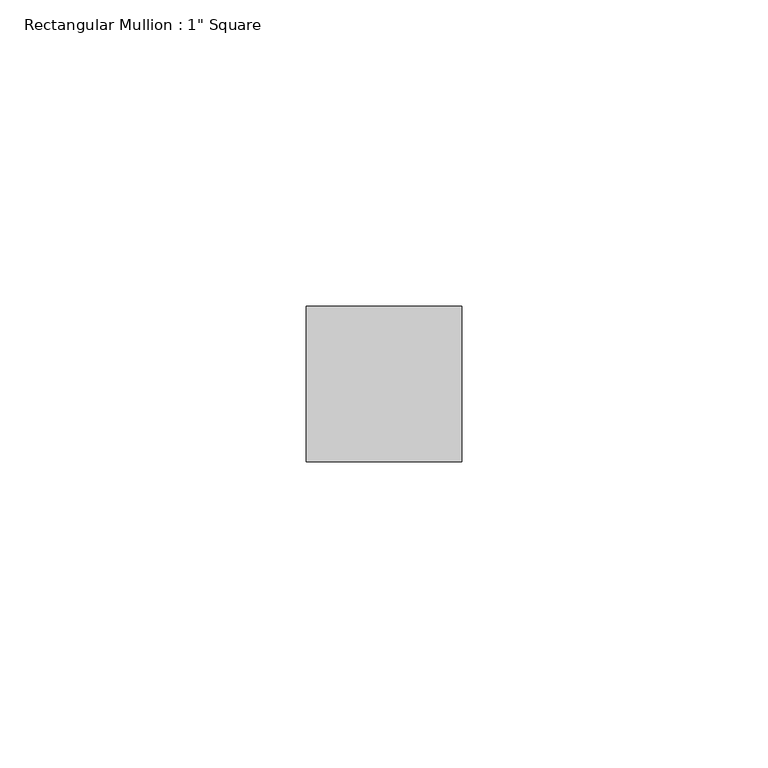
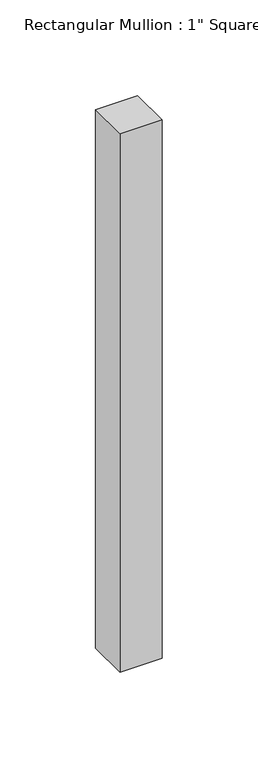
"""IFC4 building model written with IfcOpenShell, lengths in millimetres: member geometry."""

from ifc_helpers import new_model, si_unit, frame, origin, place, context, project, spatial, polyline, outline, extrude, source, transform, mapped, element, save


def member_6c57b699(model_context):
    return source(origin(), model_context, "Body", "SweptSolid", [
        extrude(outline(polyline([(12.7, 12.7), (12.7, -12.7), (-12.7, -12.7), (-12.7, 12.7), (12.7, 12.7)])), frame((0.0, 0.0, -342.9), z_axis=(0.0, 0.0, 1.0), x_axis=(1.0, 0.0, 0.0)), (0.0, 0.0, 1.0), 342.9),
    ])


if __name__ == "__main__":
    model = new_model("IFC4")
    model_context = context("Model", 3, world=origin())
    ifc_project = project(units=[si_unit("LENGTHUNIT", "METRE", prefix="MILLI")], contexts=[model_context])
    site = spatial("IfcSite", under=ifc_project)
    building = spatial("IfcBuilding", under=site)
    placement = place(None, origin())
    member_shape = member_6c57b699(model_context)
    element("IfcMember", 1, ObjectType="Rectangular Mullion : 1\" Square", at=placement, inside=building, context=model_context, shape_type="MappedRepresentation", body=[
        mapped(member_shape, transform((0.0, 0.0, 0.0), x_axis=(1.0, 0.0, 0.0), y_axis=(0.0, 1.0, 0.0), z_axis=(0.0, 0.0, 1.0))),
    ])
    save(model, "model.ifc")

# Revit data of these elements
# Type "Rectangular Mullion : 1\" Square"
#   built-in parameter 1007304 = 0.0833333 (stored number, unit not read)
#   built-in parameter 1007301 = 0.0416667 (stored number, unit not read)
#   built-in parameter 1007300 = 0.0416667 (stored number, unit not read)
